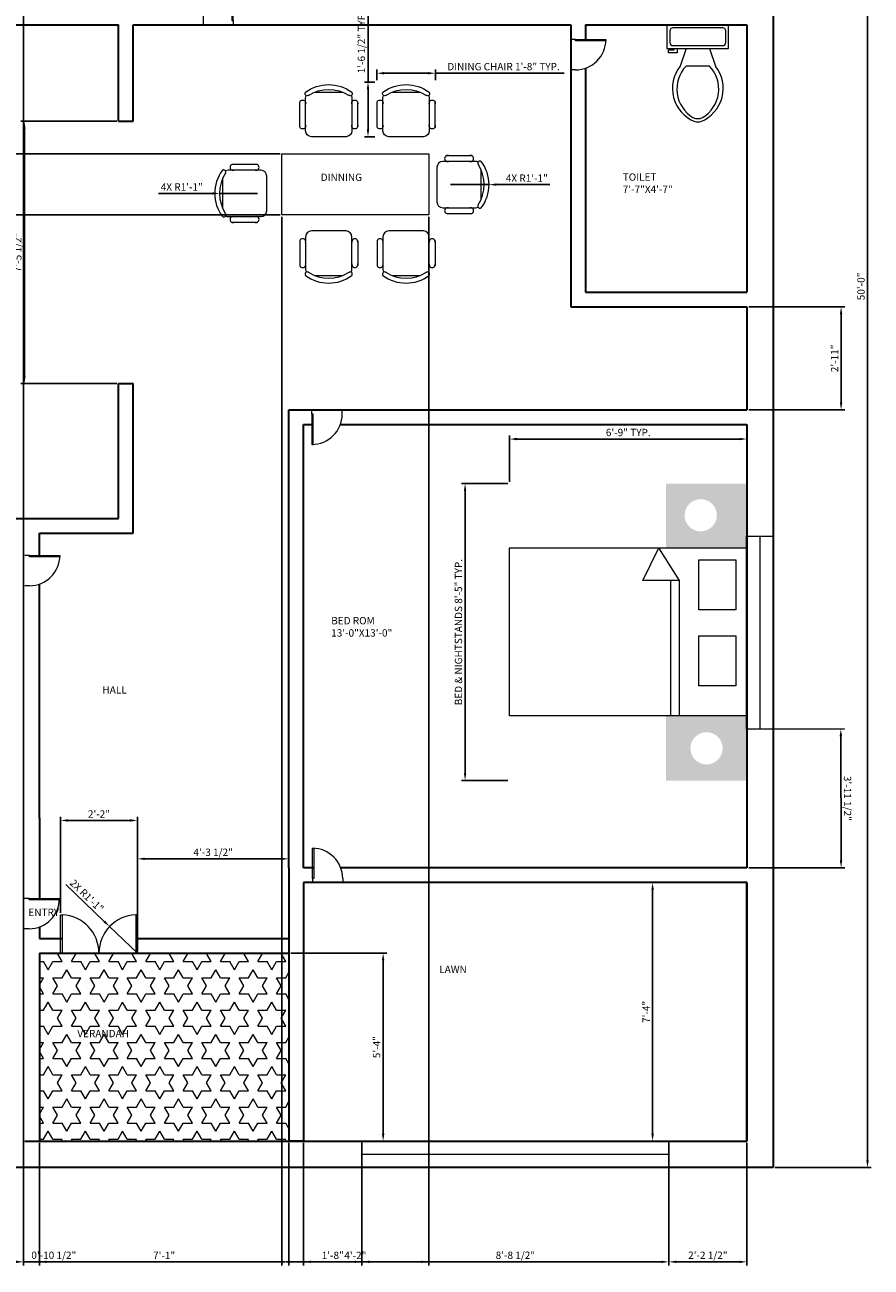
# Model space of a CAD drawing. Units: inches. Extents: x 311 to 793, y -3602 to -2932.
# Tile 2 of 3: x 505 to 793, y -3602 to -3179. Entities that reach past the tile are written whole.
import ezdxf

# ---------------------------------------------------------------- set-up
doc = ezdxf.new("R2010")
doc.units = ezdxf.units.IN
for name, color, linetype, lineweight in [('A-ANNO-DIMS', 2, 'Continuous', 18), ('A-AREA-IDEN', 7, 'Continuous', 18), ('A-DOOR', 3, 'Continuous', 18), ('A-FLOR-FIXT', 9, 'Continuous', 18), ('A-FURN', 8, 'Continuous', 18), ('A-GLAZ', 4, 'Continuous', 18), ('A-WALL', 7, 'Continuous', 35)]:
    doc.layers.add(name, color=color, linetype=linetype, lineweight=lineweight)
doc.layers.add('A-FLOR-PATT', color=116, linetype='Continuous', lineweight=13, true_color=0x136734)
doc.styles.get("Standard").update_dxf_attribs({"font": 'arial.ttf'})
doc.dimstyles.new('ISO-25', dxfattribs={"dimtxt": 2.5, "dimasz": 2.5, "dimexe": 1.25, "dimexo": 0.625, "dimtad": 1, "dimlunit": 3, "dimtxsty": 'Standard', "dimcen": 2.5, "dimadec": 0, "dimazin": 0, "dimtfac": 1, "dimtmove": 0, "dimatfit": 3, "dimfxl": 1, "dimarcsym": 0})

# ---------------------------------------------------------------- blocks, each defined once
blk = doc.blocks.new('*U5')
for p, q in [((0, 0), (0, -6)), ((-40, 0), (-40, -6))]:
    blk.add_line(p, q)
blk.add_lwpolyline([(0, 0), (0, 40), (-1.75, 40), (-1.75, 0)], close=True)
blk.add_arc((0, 0), 40, 90, 180)
blk = doc.blocks.new('*U4')
for p, q in [((0, 0), (0, 6)), ((40, 0), (40, 6))]:
    blk.add_line(p, q)
blk.add_lwpolyline([(0, 0), (0, -40), (1.75, -40), (1.75, 0)], close=True)
blk.add_arc((0, 0), 40, 270, 0)
blk = doc.blocks.new('*U2')
for p, q in [((0, 0), (0, -6)), ((40, 0), (40, -6))]:
    blk.add_line(p, q)
blk.add_lwpolyline([(0, 0), (0, 40), (1.75, 40), (1.75, 0)], close=True)
blk.add_arc((0, 0), 40, 0, 90)
blk = doc.blocks.new('DR-69P')
for points in [[(1.5, 0), (0, 0), (0, 34.5), (1.5, 34.5)], [(67.5, 0), (69, 0), (69, 34.5), (67.5, 34.5)]]:
    blk.add_lwpolyline(points, close=True)
for centre, start, end in [((0, 0), 0, 87.5104), ((69, 0), 92.4896, 180)]:
    blk.add_arc(centre, 34.5, start, end)
blk = doc.blocks.new('CHAIR7')
for p, q in [((5.12, 15.04), (17.88, 15.04)), ((0, 9), (0, -9)), ((20, 12), (3, 12)), ((23, -7.44), (23, 7.44)), ((3, -12), (20, -12)), ((5.12, -15), (17.88, -15))]:
    blk.add_line(p, q)
for centre, radius, start, end in [((5.56, 13.54), 1.56, 73.7398, 286.2602), ((17.44, 13.54), 1.56, 253.7398, 106.2602), ((3, 9), 3, 90, 180), ((20, 9), 3, 62.41556, 90), ((22.34, 11.12), 1.1, 53.30994, 212.02741), ((4.82, 0), 19.64, 327.57575, 32.42425), ((7, 0), 20, 323.1301, 36.8699), ((3, -9), 3, 180, 270), ((5.56, -13.5), 1.56, 73.7398, 286.2602), ((17.44, -13.5), 1.56, 253.7398, 106.2602), ((20, -9), 3, 270, 297.58444), ((22.34, -11.12), 1.1, 147.97259, 306.69006)]:
    blk.add_arc(centre, radius, start, end)
blk = doc.blocks.new('*U8')
for p, q in [((9.5, -6), (9.5, -2)), ((-8, -8.5), (-8, -8)), ((-7, -8), (-7, -9.5)), ((-4, -8), (-6, -14)), ((4, -8), (6, -14)), ((-10, -8.5), (-8, -8.5)), ((-10, -9.5), (-10, -8.5)), ((-7, -9.5), (-10, -9.5)), ((4, -14), (-4, -14))]:
    blk.add_line(p, q)
blk.add_lwpolyline([(10.5, -8), (10.5, 0), (-10.5, 0), (-10.5, -8)], close=True)
for points in [[(-9.5, -2), (-9.5, -6)], [(8.5, -1), (-8.5, -1)], [(-8.5, -7), (8.5, -7)]]:
    blk.add_lwpolyline(points)
for centre, radius, start, end in [((-8.62, -1.88), 0.884, 81.8699, 188.1301), ((8.62, -1.88), 0.884, 351.8699, 98.1301), ((-8.62, -6.12), 0.884, 171.8699, 278.1301), ((8.62, -6.12), 0.884, 261.8699, 8.1301), ((3.52, -21.58), 12.17, 141.4691, 247.9714), ((4.2, -21.82), 11.33, 136.3677, 238.9468), ((-3.52, -21.58), 12.17, 292.0284, 38.5307), ((-4.2, -21.82), 11.33, 301.053, 43.6321), ((0, -27.88), 4, 245.7318, 294.2682), ((0, -29), 4, 254.8605, 285.1395)]:
    blk.add_arc(centre, radius, start, end)
blk = doc.blocks.new('WINDOW-SIDE-66')
for p, q in [((0, 65.66), (9, 65.66)), ((0, 0), (0, 65.66)), ((0, 65.66), (4.5, 65.66)), ((4.5, 65.66), (4.5, 0)), ((9, 65.66), (9, 0)), ((9, 0), (0, 0))]:
    blk.add_line(p, q)
blk = doc.blocks.new('BED-DOUBLE-WITH-NIGHTSTANDS')
h = blk.add_hatch(color=256)
h.dxf.hatch_style = 1
h.set_gradient(color1=(0, 0, 255), color2=(255, 255, 0), tint=1, name='INVSPHERICAL')
h.paths.add_polyline_path([(80.82, 21.98), (53.33, 21.98), (53.33, 0), (80.82, 0)])
h.paths.add_polyline_path([(72.57, 10.99, -1), (61.59, 10.99, -1)], flags=16)
h.paths.add_polyline_path([(80.82, 101.13), (53.33, 101.13), (53.33, 79.18), (80.82, 79.18)])
h.paths.add_polyline_path([(70.59, 90.34, -1), (59.61, 90.34, -1)], flags=16)
for p, q in [((45.33, 68.14), (50.79, 79.26)), ((57.92, 68.14), (50.79, 79.26)), ((54.79, 68.14), (45.33, 68.14)), ((57.92, 68.14), (54.79, 68.14)), ((54.79, 68.14), (54.79, 22.05)), ((57.92, 22.05), (57.92, 68.14))]:
    blk.add_line(p, q)
for points in [[(0, 79.26), (80.82, 79.26), (80.82, 22.05), (0, 22.05)], [(64.46, 75.22), (77.12, 75.22), (77.12, 58.15), (64.46, 58.15)], [(64.46, 49.29), (77.12, 49.29), (77.12, 32.22), (64.46, 32.22)]]:
    blk.add_lwpolyline(points, close=True)
blk = doc.blocks.new('*D16')
at = {"layer": 'A-ANNO-DIMS', "color": 0, "lineweight": -2, "transparency": 16777216}
for p, q in [((624.73, -3197.43), (624.73, -3193.81)), ((627.23, -3195.06), (642.21, -3195.06)), ((644.71, -3197.43), (644.71, -3193.81)), ((644.71, -3195.06), (688.61, -3195.06))]:
    blk.add_line(p, q, dxfattribs=at)
at = {"layer": 'A-ANNO-DIMS', "color": 0, "transparency": 16777216}
for points in [[(627.23, -3194.64), (627.23, -3195.47), (624.73, -3195.06)], [(642.21, -3194.64), (642.21, -3195.47), (644.71, -3195.06)]]:
    blk.add_solid(points, dxfattribs=at)
at = {"layer": 'Defpoints', "color": 0, "transparency": 16777216}
for p in [(644.71, -3195.06), (624.73, -3198.05), (644.71, -3198.05)]:
    blk.add_point(p, dxfattribs=at)
at = {"layer": 'A-ANNO-DIMS', "color": 0, "transparency": 16777216, "insert": (667.91, -3193.14), "char_height": 2.5, "attachment_point": 5}
blk.add_mtext('DINING CHAIR 1\'-8" TYP.', dxfattribs=at)
blk = doc.blocks.new('*D17')
at = {"layer": 'A-ANNO-DIMS', "color": 0, "lineweight": -2, "transparency": 16777216}
for p, q in [((621.74, -3198.05), (621.74, -3173.47)), ((624.11, -3198.05), (620.49, -3198.05)), ((621.74, -3214.16), (621.74, -3200.55)), ((624.11, -3216.66), (620.49, -3216.66))]:
    blk.add_line(p, q, dxfattribs=at)
at = {"layer": 'A-ANNO-DIMS', "color": 0, "transparency": 16777216}
for points in [[(621.32, -3200.55), (622.15, -3200.55), (621.74, -3198.05)], [(621.32, -3214.16), (622.15, -3214.16), (621.74, -3216.66)]]:
    blk.add_solid(points, dxfattribs=at)
at = {"layer": 'Defpoints', "color": 0, "transparency": 16777216}
for p in [(621.74, -3198.05), (624.73, -3198.05), (624.73, -3216.66)]:
    blk.add_point(p, dxfattribs=at)
at = {"layer": 'A-ANNO-DIMS', "color": 0, "transparency": 16777216, "insert": (619.82, -3184.51), "char_height": 2.5, "attachment_point": 5, "rotation": 90}
blk.add_mtext('1\'-6 1/2" TYP.', dxfattribs=at)
blk = doc.blocks.new('*D22')
at = {"layer": 'A-ANNO-DIMS', "color": 0, "lineweight": -2, "transparency": 16777216}
for p, q in [((669.35, -3334.76), (653.56, -3334.76)), ((654.81, -3433.39), (654.81, -3337.26)), ((669.35, -3435.89), (653.56, -3435.89))]:
    blk.add_line(p, q, dxfattribs=at)
at = {"layer": 'A-ANNO-DIMS', "color": 0, "transparency": 16777216}
for points in [[(654.39, -3337.26), (655.22, -3337.26), (654.81, -3334.76)], [(654.39, -3433.39), (655.22, -3433.39), (654.81, -3435.89)]]:
    blk.add_solid(points, dxfattribs=at)
at = {"layer": 'Defpoints', "color": 0, "transparency": 16777216}
for p in [(654.81, -3334.76), (669.98, -3334.76), (669.98, -3435.89)]:
    blk.add_point(p, dxfattribs=at)
at = {"layer": 'A-ANNO-DIMS', "color": 0, "transparency": 16777216, "insert": (652.88, -3385.33), "char_height": 2.5, "attachment_point": 5, "rotation": 90}
blk.add_mtext('BED & NIGHTSTANDS 8\'-5" TYP.', dxfattribs=at)
blk = doc.blocks.new('*D23')
at = {"layer": 'A-ANNO-DIMS', "color": 0, "lineweight": -2, "transparency": 16777216}
for p, q in [((669.98, -3334.14), (669.98, -3318.35)), ((672.48, -3319.6), (748.3, -3319.6)), ((750.8, -3334.14), (750.8, -3318.35))]:
    blk.add_line(p, q, dxfattribs=at)
at = {"layer": 'A-ANNO-DIMS', "color": 0, "transparency": 16777216}
for points in [[(672.48, -3319.18), (672.48, -3320.01), (669.98, -3319.6)], [(748.3, -3319.18), (748.3, -3320.01), (750.8, -3319.6)]]:
    blk.add_solid(points, dxfattribs=at)
at = {"layer": 'Defpoints', "color": 0, "transparency": 16777216}
for p in [(750.8, -3319.6), (669.98, -3334.76), (750.8, -3334.76)]:
    blk.add_point(p, dxfattribs=at)
at = {"layer": 'A-ANNO-DIMS', "color": 0, "transparency": 16777216, "insert": (710.39, -3317.69), "char_height": 2.5, "attachment_point": 5}
blk.add_mtext('6\'-9" TYP.', dxfattribs=at)
blk = doc.blocks.new('*D24')
at = {"layer": 'A-ANNO-DIMS', "color": 0, "lineweight": -2, "transparency": 16777216}
for p, q in [((760.42, -2967.63), (793.14, -2967.63)), ((791.89, -2970.13), (791.89, -3565.13)), ((760.42, -3567.63), (793.14, -3567.63))]:
    blk.add_line(p, q, dxfattribs=at)
at = {"layer": 'A-ANNO-DIMS', "color": 0, "transparency": 16777216}
for points in [[(791.47, -2970.13), (792.31, -2970.13), (791.89, -2967.63)], [(791.47, -3565.13), (792.31, -3565.13), (791.89, -3567.63)]]:
    blk.add_solid(points, dxfattribs=at)
at = {"layer": 'Defpoints', "color": 0, "transparency": 16777216}
for p in [(759.79, -2967.63), (759.79, -3567.63), (791.89, -3567.63)]:
    blk.add_point(p, dxfattribs=at)
at = {"layer": 'A-ANNO-DIMS', "color": 0, "transparency": 16777216, "insert": (789.99, -3267.63), "char_height": 2.5, "attachment_point": 5, "rotation": 90}
blk.add_mtext('50\'-0"', dxfattribs=at)
blk = doc.blocks.new('*D26')
at = {"layer": 'A-ANNO-DIMS', "color": 0, "lineweight": -2, "transparency": 16777216}
for p, q in [((509.79, -3559.25), (509.79, -3600.98)), ((594.79, -3559.25), (594.79, -3600.98)), ((512.29, -3599.73), (592.29, -3599.73))]:
    blk.add_line(p, q, dxfattribs=at)
at = {"layer": 'A-ANNO-DIMS', "color": 0, "transparency": 16777216}
for points in [[(512.29, -3599.31), (512.29, -3600.14), (509.79, -3599.73)], [(592.29, -3599.31), (592.29, -3600.14), (594.79, -3599.73)]]:
    blk.add_solid(points, dxfattribs=at)
at = {"layer": 'Defpoints', "color": 0, "transparency": 16777216}
for p in [(509.79, -3558.63), (594.79, -3558.63), (594.79, -3599.73)]:
    blk.add_point(p, dxfattribs=at)
at = {"layer": 'A-ANNO-DIMS', "color": 0, "transparency": 16777216, "insert": (552.29, -3597.85), "char_height": 2.5, "attachment_point": 5}
blk.add_mtext('7\'-1"', dxfattribs=at)
blk = doc.blocks.new('*D27')
at = {"layer": 'A-ANNO-DIMS', "color": 0, "lineweight": -2, "transparency": 16777216}
for p, q in [((599.79, -3559.25), (599.79, -3600.98)), ((619.66, -3559.25), (619.66, -3600.98)), ((602.29, -3599.73), (617.16, -3599.73))]:
    blk.add_line(p, q, dxfattribs=at)
at = {"layer": 'A-ANNO-DIMS', "color": 0, "transparency": 16777216}
for points in [[(602.29, -3599.31), (602.29, -3600.14), (599.79, -3599.73)], [(617.16, -3599.31), (617.16, -3600.14), (619.66, -3599.73)]]:
    blk.add_solid(points, dxfattribs=at)
at = {"layer": 'Defpoints', "color": 0, "transparency": 16777216}
for p in [(599.79, -3558.63), (619.66, -3558.63), (619.66, -3599.73)]:
    blk.add_point(p, dxfattribs=at)
at = {"layer": 'A-ANNO-DIMS', "color": 0, "transparency": 16777216, "insert": (609.73, -3597.82), "char_height": 2.5, "attachment_point": 5}
blk.add_mtext('1\'-8"', dxfattribs=at)
blk = doc.blocks.new('*D28')
at = {"layer": 'A-ANNO-DIMS', "color": 0, "lineweight": -2, "transparency": 16777216}
for p, q in [((619.66, -3559.25), (619.66, -3600.98)), ((724.22, -3559.25), (724.22, -3600.98)), ((622.16, -3599.73), (721.72, -3599.73))]:
    blk.add_line(p, q, dxfattribs=at)
at = {"layer": 'A-ANNO-DIMS', "color": 0, "transparency": 16777216}
for points in [[(622.16, -3599.31), (622.16, -3600.14), (619.66, -3599.73)], [(721.72, -3599.31), (721.72, -3600.14), (724.22, -3599.73)]]:
    blk.add_solid(points, dxfattribs=at)
at = {"layer": 'Defpoints', "color": 0, "transparency": 16777216}
for p in [(619.66, -3558.63), (724.22, -3558.63), (724.22, -3599.73)]:
    blk.add_point(p, dxfattribs=at)
at = {"layer": 'A-ANNO-DIMS', "color": 0, "transparency": 16777216, "insert": (671.94, -3597.81), "char_height": 2.5, "attachment_point": 5}
blk.add_mtext('8\'-8 1/2"', dxfattribs=at)
blk = doc.blocks.new('*D29')
at = {"layer": 'A-ANNO-DIMS', "color": 0, "lineweight": -2, "transparency": 16777216}
for p, q in [((724.22, -3559.25), (724.22, -3600.98)), ((750.79, -3559.25), (750.79, -3600.98)), ((726.72, -3599.73), (748.29, -3599.73))]:
    blk.add_line(p, q, dxfattribs=at)
at = {"layer": 'A-ANNO-DIMS', "color": 0, "transparency": 16777216}
for points in [[(726.72, -3599.31), (726.72, -3600.14), (724.22, -3599.73)], [(748.29, -3599.31), (748.29, -3600.14), (750.79, -3599.73)]]:
    blk.add_solid(points, dxfattribs=at)
at = {"layer": 'Defpoints', "color": 0, "transparency": 16777216}
for p in [(724.22, -3558.63), (750.79, -3558.63), (750.79, -3599.73)]:
    blk.add_point(p, dxfattribs=at)
at = {"layer": 'A-ANNO-DIMS', "color": 0, "transparency": 16777216, "insert": (737.5, -3597.81), "char_height": 2.5, "attachment_point": 5}
blk.add_mtext('2\'-2 1/2"', dxfattribs=at)
blk = doc.blocks.new('*D30')
at = {"layer": 'A-ANNO-DIMS', "color": 0, "lineweight": -2, "transparency": 16777216}
for p, q in [((750.17, -3470.63), (717.44, -3470.63)), ((718.69, -3556.13), (718.69, -3473.13)), ((750.17, -3558.63), (717.44, -3558.63))]:
    blk.add_line(p, q, dxfattribs=at)
at = {"layer": 'A-ANNO-DIMS', "color": 0, "transparency": 16777216}
for points in [[(718.27, -3473.13), (719.11, -3473.13), (718.69, -3470.63)], [(718.27, -3556.13), (719.11, -3556.13), (718.69, -3558.63)]]:
    blk.add_solid(points, dxfattribs=at)
at = {"layer": 'Defpoints', "color": 0, "transparency": 16777216}
for p in [(718.69, -3470.63), (750.79, -3470.63), (750.79, -3558.63)]:
    blk.add_point(p, dxfattribs=at)
at = {"layer": 'A-ANNO-DIMS', "color": 0, "transparency": 16777216, "insert": (716.82, -3514.63), "char_height": 2.5, "attachment_point": 5, "rotation": 90}
blk.add_mtext('7\'-4"', dxfattribs=at)
blk = doc.blocks.new('*D31')
at = {"layer": 'A-ANNO-DIMS', "color": 0, "lineweight": -2, "transparency": 16777216}
for p, q in [((595.42, -3494.63), (628.14, -3494.63)), ((626.89, -3497.13), (626.89, -3556.13)), ((595.42, -3558.63), (628.14, -3558.63))]:
    blk.add_line(p, q, dxfattribs=at)
at = {"layer": 'A-ANNO-DIMS', "color": 0, "transparency": 16777216}
for points in [[(626.47, -3497.13), (627.31, -3497.13), (626.89, -3494.63)], [(626.47, -3556.13), (627.31, -3556.13), (626.89, -3558.63)]]:
    blk.add_solid(points, dxfattribs=at)
at = {"layer": 'Defpoints', "color": 0, "transparency": 16777216}
for p in [(594.79, -3494.63), (594.79, -3558.63), (626.89, -3558.63)]:
    blk.add_point(p, dxfattribs=at)
at = {"layer": 'A-ANNO-DIMS', "color": 0, "transparency": 16777216, "insert": (624.99, -3526.63), "char_height": 2.5, "attachment_point": 5, "rotation": 90}
blk.add_mtext('5\'-4"', dxfattribs=at)
blk = doc.blocks.new('*D41')
at = {"layer": 'A-ANNO-DIMS', "color": 0, "lineweight": -2, "transparency": 16777216}
for p, q in [((517.01, -3480.92), (517.01, -3448.2)), ((519.51, -3449.45), (540.67, -3449.45)), ((543.17, -3480.92), (543.17, -3448.2))]:
    blk.add_line(p, q, dxfattribs=at)
at = {"layer": 'A-ANNO-DIMS', "color": 0, "transparency": 16777216}
for points in [[(519.51, -3449.03), (519.51, -3449.86), (517.01, -3449.45)], [(540.67, -3449.03), (540.67, -3449.86), (543.17, -3449.45)]]:
    blk.add_solid(points, dxfattribs=at)
at = {"layer": 'Defpoints', "color": 0, "transparency": 16777216}
for p in [(543.17, -3449.45), (517.01, -3481.55), (543.17, -3481.55)]:
    blk.add_point(p, dxfattribs=at)
at = {"layer": 'A-ANNO-DIMS', "color": 0, "transparency": 16777216, "insert": (530.09, -3447.57), "char_height": 2.5, "attachment_point": 5}
blk.add_mtext('2\'-2"', dxfattribs=at)
blk = doc.blocks.new('*D44')
at = {"layer": 'A-ANNO-DIMS', "color": 0, "lineweight": -2, "transparency": 16777216}
for p, q in [((751.33, -3418.35), (784.06, -3418.29)), ((782.81, -3420.79), (782.89, -3463.07)), ((751.42, -3465.62), (784.14, -3465.57))]:
    blk.add_line(p, q, dxfattribs=at)
at = {"layer": 'A-ANNO-DIMS', "color": 0, "transparency": 16777216}
for points in [[(783.23, -3420.79), (782.39, -3420.79), (782.81, -3418.29)], [(783.3, -3463.07), (782.47, -3463.07), (782.89, -3465.57)]]:
    blk.add_solid(points, dxfattribs=at)
at = {"layer": 'Defpoints', "color": 0, "transparency": 16777216}
for p in [(750.71, -3418.35), (750.79, -3465.63), (782.89, -3465.57)]:
    blk.add_point(p, dxfattribs=at)
at = {"layer": 'A-ANNO-DIMS', "color": 0, "transparency": 16777216, "insert": (784.77, -3441.93), "char_height": 2.5, "attachment_point": 5, "rotation": 270.1016}
blk.add_mtext('3\'-11 1/2"', dxfattribs=at)
blk = doc.blocks.new('*D45')
at = {"layer": 'A-ANNO-DIMS', "color": 0, "lineweight": -2, "transparency": 16777216}
for p, q in [((592.43, -3243.92), (592.43, -3600.98)), ((642.43, -3243.92), (642.43, -3600.98)), ((639.93, -3599.73), (594.93, -3599.73))]:
    blk.add_line(p, q, dxfattribs=at)
at = {"layer": 'A-ANNO-DIMS', "color": 0, "transparency": 16777216}
for points in [[(594.93, -3599.31), (594.93, -3600.14), (592.43, -3599.73)], [(639.93, -3599.31), (639.93, -3600.14), (642.43, -3599.73)]]:
    blk.add_solid(points, dxfattribs=at)
at = {"layer": 'Defpoints', "color": 0, "transparency": 16777216}
for p in [(592.43, -3243.3), (642.43, -3243.3), (592.43, -3599.73)]:
    blk.add_point(p, dxfattribs=at)
at = {"layer": 'A-ANNO-DIMS', "color": 0, "transparency": 16777216, "insert": (617.43, -3597.85), "char_height": 2.5, "attachment_point": 5}
blk.add_mtext('4\'-2"', dxfattribs=at)
blk = doc.blocks.new('*D46')
at = {"layer": 'A-ANNO-DIMS', "color": 0, "lineweight": -2, "transparency": 16777216}
for p, q in [((591.8, -3222.54), (315.44, -3222.54)), ((316.69, -3240.8), (316.69, -3225.04)), ((591.8, -3243.3), (315.44, -3243.3))]:
    blk.add_line(p, q, dxfattribs=at)
at = {"layer": 'A-ANNO-DIMS', "color": 0, "transparency": 16777216}
for points in [[(316.27, -3225.04), (317.11, -3225.04), (316.69, -3222.54)], [(316.27, -3240.8), (317.11, -3240.8), (316.69, -3243.3)]]:
    blk.add_solid(points, dxfattribs=at)
at = {"layer": 'Defpoints', "color": 0, "transparency": 16777216}
for p in [(316.69, -3222.54), (592.43, -3222.54), (592.43, -3243.3)]:
    blk.add_point(p, dxfattribs=at)
at = {"layer": 'A-ANNO-DIMS', "color": 0, "transparency": 16777216, "insert": (314.79, -3232.92), "char_height": 2.5, "attachment_point": 5, "rotation": 90}
blk.add_mtext('1\'-9"', dxfattribs=at)
blk = doc.blocks.new('*D50')
at = {"layer": 'A-ANNO-DIMS', "color": 0, "lineweight": -2, "transparency": 16777216}
for p, q in [((494.06, -3042.22), (494.06, -3600.98)), ((504.38, -3042.22), (504.38, -3600.98)), ((496.56, -3599.73), (501.88, -3599.73)), ((504.38, -3599.73), (522.54, -3599.73))]:
    blk.add_line(p, q, dxfattribs=at)
at = {"layer": 'A-ANNO-DIMS', "color": 0, "transparency": 16777216}
for points in [[(496.56, -3599.31), (496.56, -3600.14), (494.06, -3599.73)], [(501.88, -3599.31), (501.88, -3600.14), (504.38, -3599.73)]]:
    blk.add_solid(points, dxfattribs=at)
at = {"layer": 'Defpoints', "color": 0, "transparency": 16777216}
for p in [(494.06, -3041.59), (504.38, -3041.59), (504.38, -3599.73)]:
    blk.add_point(p, dxfattribs=at)
at = {"layer": 'A-ANNO-DIMS', "color": 0, "transparency": 16777216, "insert": (514.71, -3597.81), "char_height": 2.5, "attachment_point": 5}
blk.add_mtext('0\'-10 1/2"', dxfattribs=at)
blk = doc.blocks.new('*D52')
at = {"layer": 'A-ANNO-DIMS', "color": 0, "lineweight": -2, "transparency": 16777216}
for p, q in [((543.17, -3494), (543.17, -3461.28)), ((545.67, -3462.53), (592.29, -3462.53)), ((594.79, -3494), (594.79, -3461.28))]:
    blk.add_line(p, q, dxfattribs=at)
at = {"layer": 'A-ANNO-DIMS', "color": 0, "transparency": 16777216}
for points in [[(545.67, -3462.11), (545.67, -3462.94), (543.17, -3462.53)], [(592.29, -3462.11), (592.29, -3462.94), (594.79, -3462.53)]]:
    blk.add_solid(points, dxfattribs=at)
at = {"layer": 'Defpoints', "color": 0, "transparency": 16777216}
for p in [(594.79, -3462.53), (543.17, -3494.63), (594.79, -3494.63)]:
    blk.add_point(p, dxfattribs=at)
at = {"layer": 'A-ANNO-DIMS', "color": 0, "transparency": 16777216, "insert": (568.98, -3460.61), "char_height": 2.5, "attachment_point": 5}
blk.add_mtext('4\'-3 1/2"', dxfattribs=at)
blk = doc.blocks.new('*D53')
at = {"layer": 'A-ANNO-DIMS', "color": 0, "lineweight": -2, "transparency": 16777216}
for p, q in [((536.17, -3211.42), (503.44, -3211.42)), ((504.69, -3298.24), (504.69, -3213.92)), ((536.17, -3300.74), (503.44, -3300.74))]:
    blk.add_line(p, q, dxfattribs=at)
at = {"layer": 'A-ANNO-DIMS', "color": 0, "transparency": 16777216}
for points in [[(504.27, -3213.92), (505.11, -3213.92), (504.69, -3211.42)], [(504.27, -3298.24), (505.11, -3298.24), (504.69, -3300.74)]]:
    blk.add_solid(points, dxfattribs=at)
at = {"layer": 'Defpoints', "color": 0, "transparency": 16777216}
for p in [(504.69, -3211.42), (536.79, -3211.42), (536.79, -3300.74)]:
    blk.add_point(p, dxfattribs=at)
at = {"layer": 'A-ANNO-DIMS', "color": 0, "transparency": 16777216, "insert": (502.77, -3256.08), "char_height": 2.5, "attachment_point": 5, "rotation": 90}
blk.add_mtext('7\'-5 1/2"', dxfattribs=at)
blk = doc.blocks.new('*D54')
at = {"layer": 'A-ANNO-DIMS', "color": 0, "lineweight": -2, "transparency": 16777216}
for p, q in [((751.42, -3274.63), (784.14, -3274.63)), ((782.89, -3277.13), (782.89, -3307.13)), ((751.42, -3309.63), (784.14, -3309.63))]:
    blk.add_line(p, q, dxfattribs=at)
at = {"layer": 'A-ANNO-DIMS', "color": 0, "transparency": 16777216}
for points in [[(782.47, -3277.13), (783.31, -3277.13), (782.89, -3274.63)], [(782.47, -3307.13), (783.31, -3307.13), (782.89, -3309.63)]]:
    blk.add_solid(points, dxfattribs=at)
at = {"layer": 'Defpoints', "color": 0, "transparency": 16777216}
for p in [(750.79, -3274.63), (750.79, -3309.63), (782.89, -3309.63)]:
    blk.add_point(p, dxfattribs=at)
at = {"layer": 'A-ANNO-DIMS', "color": 0, "transparency": 16777216, "insert": (781.01, -3292.13), "char_height": 2.5, "attachment_point": 5, "rotation": 90}
blk.add_mtext('2\'-11"', dxfattribs=at)
blk = doc.blocks.new('*D55')
at = {"layer": 'A-ANNO-DIMS', "color": 0, "lineweight": -2, "transparency": 16777216}
for p, q in [((518.77, -3471.26), (531.92, -3483.85)), ((543.17, -3494.63), (533.72, -3485.58))]:
    blk.add_line(p, q, dxfattribs=at)
at = {"layer": 'A-ANNO-DIMS', "color": 0, "transparency": 16777216}
blk.add_solid([(532.2, -3483.55), (531.63, -3484.15), (533.72, -3485.58)], dxfattribs=at)
at = {"layer": 'Defpoints', "color": 0, "transparency": 16777216}
for p in [(533.72, -3485.58), (543.17, -3494.63)]:
    blk.add_point(p, dxfattribs=at)
at = {"layer": 'A-ANNO-DIMS', "color": 0, "transparency": 16777216, "insert": (525.74, -3475.33), "char_height": 2.5, "attachment_point": 5, "rotation": 316.245}
blk.add_mtext('2X R1\'-1"', dxfattribs=at)
blk = doc.blocks.new('*D56')
at = {"layer": 'A-ANNO-DIMS', "color": 0, "lineweight": -2, "transparency": 16777216}
for p, q in [((649.82, -3232.98), (662.96, -3232.98)), ((683.72, -3232.98), (665.46, -3232.98))]:
    blk.add_line(p, q, dxfattribs=at)
at = {"layer": 'A-ANNO-DIMS', "color": 0, "transparency": 16777216}
blk.add_solid([(665.46, -3232.57), (665.46, -3233.4), (662.96, -3232.98)], dxfattribs=at)
at = {"layer": 'Defpoints', "color": 0, "transparency": 16777216}
for p in [(649.82, -3232.98), (662.96, -3232.98)]:
    blk.add_point(p, dxfattribs=at)
at = {"layer": 'A-ANNO-DIMS', "color": 0, "transparency": 16777216, "insert": (675.84, -3231.1), "char_height": 2.5, "attachment_point": 5, "rotation": 359.9994}
blk.add_mtext('4X R1\'-1"', dxfattribs=at)
blk = doc.blocks.new('*D57')
at = {"layer": 'A-ANNO-DIMS', "color": 0, "lineweight": -2, "transparency": 16777216}
for p, q in [((550.41, -3235.98), (568.68, -3235.98)), ((584.08, -3235.98), (571.18, -3235.98))]:
    blk.add_line(p, q, dxfattribs=at)
at = {"layer": 'A-ANNO-DIMS', "color": 0, "transparency": 16777216}
blk.add_solid([(568.68, -3235.57), (568.68, -3236.4), (571.18, -3235.98)], dxfattribs=at)
at = {"layer": 'Defpoints', "color": 0, "transparency": 16777216}
for p in [(571.18, -3235.98), (584.08, -3235.98)]:
    blk.add_point(p, dxfattribs=at)
at = {"layer": 'A-ANNO-DIMS', "color": 0, "transparency": 16777216, "insert": (558.3, -3234.1), "char_height": 2.5, "attachment_point": 5, "rotation": 0.0014}
blk.add_mtext('4X R1\'-1"', dxfattribs=at)

msp = doc.modelspace()

# ---------------------------------------------------------------- hatches: boundary and pattern name
at = {"layer": 'A-FLOR-PATT'}
h = msp.add_hatch(dxfattribs=at)
h.set_pattern_fill('STARS', color=256)
h.paths.add_polyline_path([(594.791, -3494.626), (509.791, -3494.626), (509.791, -3558.626), (594.791, -3558.626)])
h.paths.add_polyline_path([(522.078, -3524.626), (542.734, -3524.626), (542.734, -3519.474), (522.078, -3519.474)], flags=24)

# ---------------------------------------------------------------- linework, layer by layer
at = {"layer": 'A-FURN'}
msp.add_lwpolyline([(592.429, -3222.538), (642.428, -3222.538), (642.428, -3243.296), (592.429, -3243.296)], close=True, dxfattribs=at)
at = {"layer": 'A-GLAZ'}
for p, q in [((619.662, -3558.626), (619.662, -3567.626)), ((724.218, -3567.626), (724.218, -3558.626)), ((724.218, -3558.626), (724.218, -3563.126)), ((724.218, -3563.126), (619.662, -3563.126)), ((619.662, -3567.626), (724.218, -3567.626))]:
    msp.add_line(p, q, dxfattribs=at)
at = {"layer": 'A-WALL'}
for p, q in [((759.791, -2967.626), (759.791, -3567.626)), ((408.791, -3178.626), (536.791, -3178.626)), ((536.791, -3211.417), (536.791, -3178.626)), ((541.791, -3178.626), (690.791, -3178.626)), ((541.791, -3211.417), (541.791, -3178.626)), ((690.791, -3178.626), (690.791, -3274.626)), ((695.791, -3178.626), (695.791, -3184.055)), ((695.791, -3178.626), (750.791, -3178.626)), ((750.791, -3178.626), (750.791, -3269.626)), ((695.791, -3193.368), (695.791, -3269.626)), ((536.791, -3211.417), (541.791, -3211.417)), ((695.791, -3269.626), (750.791, -3269.626)), ((690.791, -3274.626), (750.791, -3274.626)), ((750.791, -3274.626), (750.791, -3309.626)), ((536.791, -3346.626), (536.791, -3300.744)), ((536.791, -3300.744), (541.791, -3300.744)), ((541.791, -3351.626), (541.791, -3300.744)), ((594.791, -3465.626), (594.791, -3309.626)), ((594.791, -3309.626), (603.074, -3309.626)), ((594.791, -3309.626), (750.791, -3309.626)), ((599.791, -3465.626), (599.791, -3314.626)), ((599.791, -3314.626), (603.074, -3314.626)), ((612.33, -3314.626), (750.791, -3314.626)), ((750.791, -3314.626), (750.791, -3465.626)), ((408.791, -3346.626), (536.791, -3346.626)), ((509.791, -3351.626), (541.791, -3351.626)), ((509.791, -3359.689), (509.791, -3351.626)), ((509.791, -3386.89), (509.791, -3369.001)), ((509.791, -3448.626), (509.791, -3386.89)), ((509.791, -3448.626), (509.791, -3476.441)), ((594.791, -3465.626), (594.791, -3494.626)), ((603.243, -3465.626), (599.791, -3465.626)), ((750.791, -3465.626), (612.467, -3465.626)), ((750.791, -3470.626), (599.791, -3470.626)), ((599.791, -3470.626), (599.791, -3558.626)), ((750.791, -3558.626), (750.791, -3470.626)), ((750.791, -3470.626), (750.791, -3558.626)), ((509.791, -3485.705), (509.791, -3489.626)), ((509.791, -3489.626), (517.581, -3489.626)), ((542.6, -3489.626), (594.791, -3489.626)), ((509.791, -3494.626), (594.791, -3494.626)), ((509.791, -3494.626), (509.791, -3558.626)), ((594.791, -3494.626), (594.791, -3558.626)), ((504.791, -3558.626), (599.791, -3558.626)), ((599.791, -3558.626), (594.791, -3558.626)), ((599.791, -3558.626), (750.791, -3558.626)), ((759.791, -3567.626), (399.791, -3567.626))]:
    msp.add_line(p, q, dxfattribs=at)

# ---------------------------------------------------------------- block references
at = {"layer": 'A-DOOR'}
for name, p, xscale, yscale, zscale in [('*U5', (575.86, -3177.104), 0.2580993088148874, 0.2580993088148874, 0.2580993088148874), ('*U4', (602.623, -3311.11), 0.2580993088148874, 0.2580993088148874, 0.2580993088148874), ('*U2', (602.791, -3469.225), 0.2580993088148874, 0.2580993088148874, 0.2580993088148874), ('DR-69P', (517.013, -3494.626), 0.3790695160026234, 0.3790695160026234, 0.3790695160026234)]:
    msp.add_blockref(name, p, dxfattribs=dict(at, xscale=xscale, yscale=yscale, zscale=zscale))
at = {"layer": 'A-DOOR', "xscale": 0.2580993088148874, "yscale": 0.2580993088148874, "zscale": 0.2580993088148874, "rotation": 270}
for p in [(692.439, -3183.603), (506.437, -3359.238), (506.298, -3475.99)]:
    msp.add_blockref('*U2', p, dxfattribs=at)
at = {"layer": 'A-FLOR-FIXT'}
msp.add_blockref('*U8', (734.087, -3178.626), dxfattribs=at)
at = {"layer": 'A-FURN', "yscale": 0.6568757526623843, "zscale": 0.6568757526623843}
for p, xscale, rotation in [((608.356, -3216.663), -0.6568757526623843, 270), ((634.709, -3216.663), -0.6568757526623843, 270), ((587.245, -3235.984), 0.6568757526623843, 180), ((608.356, -3248.769), 0.6568757526623843, 270), ((634.709, -3248.769), 0.6568757526623843, 270)]:
    msp.add_blockref('CHAIR7', p, dxfattribs=dict(at, xscale=xscale, rotation=rotation))
at = {"layer": 'A-FURN', "xscale": 0.6568757526623843, "yscale": 0.6568757526623843, "zscale": 0.6568757526623843}
msp.add_blockref('CHAIR7', (645.223, -3232.984), dxfattribs=at)
at = {"layer": 'A-FURN'}
msp.add_blockref('BED-DOUBLE-WITH-NIGHTSTANDS', (669.975, -3435.892), dxfattribs=at)
at = {"layer": 'A-GLAZ'}
msp.add_blockref('WINDOW-SIDE-66', (750.707, -3418.349), dxfattribs=at)

# ---------------------------------------------------------------- texts
at = {"layer": 'A-AREA-IDEN', "char_height": 2.5, "attachment_point": 1}
for s, width, insert in [('DINNING', 25.20231, (605.623, -3229.237)), ('TOILET\\P7\'-7"X4\'-7"', 21.07717, (708.513, -3229.149)), ('BED ROM\\P13\'-0"X13\'-0"', 32.72157, (609.203, -3380.188)), ('HALL', 30.32235, (531.282, -3403.751)), ('ENTRY', 4.47945, (506.056, -3479.492)), ('LAWN', 69.99881, (646.014, -3498.902)), ('VERANDAH', 61.79692, (522.718, -3520.761))]:
    msp.add_mtext_dynamic_manual_height_columns(s, width=width, gutter_width=12.5, heights=[0], dxfattribs=dict(at, insert=insert))

# ---------------------------------------------------------------- dimensions: what is measured, and where the dimension line sits
at = {"layer": 'A-ANNO-DIMS'}
for base, p1, p2, angle, picture, middle in [((791.891, -3567.626), (759.791, -2967.626), (759.791, -3567.626), 270, '*D24', (789.99, -3267.626)), ((504.691, -3211.417), (536.791, -3300.744), (536.791, -3211.417), 90, '*D53', (502.773, -3256.08)), ((316.691, -3222.538), (592.429, -3243.296), (592.429, -3222.538), 90, '*D46', (314.79, -3232.917)), ((782.891, -3309.626), (750.791, -3274.626), (750.791, -3309.626), 270, '*D54', (781.011, -3292.126)), ((782.891, -3465.569), (750.707, -3418.349), (750.791, -3465.626), 270.10161, '*D44', (784.767, -3441.927)), ((718.691, -3470.626), (750.791, -3558.626), (750.791, -3470.626), 90, '*D30', (716.816, -3514.626)), ((626.891, -3558.626), (594.791, -3494.626), (594.791, -3558.626), 270, '*D31', (624.995, -3526.626))]:
    dim = msp.add_linear_dim(base=base, p1=p1, p2=p2, angle=angle, dimstyle='ISO-25', override={"dimdec": 1, "dimlfac": 1, "dimrnd": 0, "dimzin": 1, "dimdsep": 46, "dimlunit": 4, "dimfrac": 2}, dxfattribs=at)
    dim.commit()
    dim.dimension.update_dxf_attribs({"geometry": picture, "text_midpoint": middle})
for base, p1, p2, picture, middle in [((504.381, -3599.726), (494.057, -3041.593), (504.381, -3041.593), '*D50', (514.712, -3597.808)), ((592.429, -3599.726), (642.428, -3243.296), (592.429, -3243.296), '*D45', (617.429, -3597.845)), ((543.168, -3449.448), (517.013, -3481.548), (543.168, -3481.548), '*D41', (530.091, -3447.568)), ((594.791, -3462.526), (543.168, -3494.626), (594.791, -3494.626), '*D52', (568.98, -3460.607)), ((594.791, -3599.726), (509.791, -3558.626), (594.791, -3558.626), '*D26', (552.291, -3597.845)), ((619.662, -3599.726), (599.791, -3558.626), (619.662, -3558.626), '*D27', (609.726, -3597.824)), ((724.218, -3599.726), (619.662, -3558.626), (724.218, -3558.626), '*D28', (671.94, -3597.808)), ((750.791, -3599.726), (724.218, -3558.626), (750.791, -3558.626), '*D29', (737.505, -3597.808))]:
    dim = msp.add_linear_dim(base=base, p1=p1, p2=p2, dimstyle='ISO-25', override={"dimdec": 1, "dimlfac": 1, "dimrnd": 0, "dimzin": 1, "dimdsep": 46, "dimlunit": 4, "dimfrac": 2}, dxfattribs=at)
    dim.commit()
    dim.dimension.update_dxf_attribs({"geometry": picture, "text_midpoint": middle})
for base, p1, p2, text, picture, middle in [((621.737, -3198.052), (624.734, -3216.663), (624.734, -3198.052), '<> TYP.', '*D17', (619.819, -3184.512)), ((654.806, -3334.764), (669.975, -3435.892), (669.975, -3334.764), 'BED & NIGHTSTANDS <> TYP.', '*D22', (652.881, -3385.328))]:
    dim = msp.add_linear_dim(base=base, p1=p1, p2=p2, angle=90, text=text, dimstyle='ISO-25', override={"dimdec": 1, "dimlfac": 1, "dimrnd": 0, "dimzin": 1, "dimdsep": 46, "dimlunit": 4, "dimfrac": 2}, dxfattribs=at)
    dim.commit()
    dim.dimension.update_dxf_attribs({"geometry": picture, "text_midpoint": middle})
for base, p1, p2, text, picture, middle in [((644.712, -3195.055), (624.734, -3198.052), (644.712, -3198.052), 'DINING CHAIR <> TYP.', '*D16', (667.91, -3193.137)), ((750.796, -3319.595), (669.975, -3334.764), (750.796, -3334.764), '<> TYP.', '*D23', (710.386, -3317.694))]:
    dim = msp.add_linear_dim(base=base, p1=p1, p2=p2, text=text, dimstyle='ISO-25', override={"dimdec": 1, "dimlfac": 1, "dimrnd": 0, "dimzin": 1, "dimdsep": 46, "dimlunit": 4, "dimfrac": 2}, dxfattribs=at)
    dim.commit()
    dim.dimension.update_dxf_attribs({"geometry": picture, "text_midpoint": middle})
for center, mpoint, text, picture, middle in [((584.077, -3235.984), (571.176, -3235.984), '4X <>', '*D57', (558.295, -3234.103)), ((649.821, -3232.984), (662.959, -3232.984), '4X <>', '*D56', (675.839, -3231.103)), ((543.168, -3494.626), (533.722, -3485.581), '2X <>', '*D55', (525.741, -3475.335))]:
    dim = msp.add_radius_dim(center=center, mpoint=mpoint, text=text, dimstyle='ISO-25', override={"dimdec": 1, "dimlfac": 1, "dimrnd": 0, "dimzin": 1, "dimdsep": 46, "dimlunit": 4, "dimfrac": 2}, dxfattribs=at)
    dim.commit()
    dim.dimension.update_dxf_attribs({"geometry": picture, "text_midpoint": middle})

doc.saveas('drawing.dxf')
